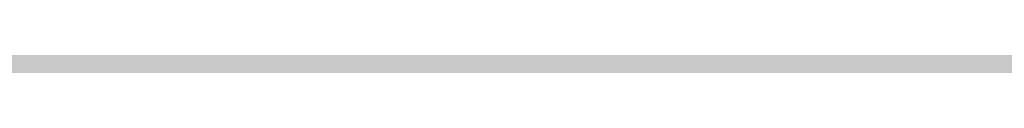
# Model space of a CAD drawing. Units: inches. Extents: x 2091 to 2899, y 967 to 2217.
# Tile 196 of 256: x 2203.18039 to 2203.25707, y 1152.24727 to 1152.24748. Entities that reach past the tile are written whole.
import ezdxf

# ---------------------------------------------------------------- set-up
doc = ezdxf.new("R2010")
doc.units = ezdxf.units.IN
doc.layers.add('A-WALL-PATT', color=141, linetype='Continuous', lineweight=13, true_color=0xadddf7)

msp = doc.modelspace()

# ---------------------------------------------------------------- hatches: boundary and pattern name
at = {"layer": 'A-WALL-PATT'}
h = msp.add_hatch(color=256, dxfattribs=at)
h.dxf.hatch_style = 1
h.paths.add_polyline_path([(2803.143603, 2050.919059), (2203.143603, 2050.919059), (2203.143603, 1090.919059), (2803.143603, 1090.919059)])
h.paths.add_polyline_path([(2635.79885, 1147.540465), (2674.524052, 1147.540465, 0.376086), (2678.529665, 1152.880202), (2678.529665, 1159.556473, 0.333335), (2674.524319, 1163.561846), (2674.524319, 1163.56185), (2674.524319, 1192.93439), (2635.805971, 1192.93439), (2597.087622, 1192.93439), (2597.087622, 1163.561846, 0.333335), (2593.082276, 1159.556473), (2593.082276, 1152.880202, 0.376086), (2597.087889, 1147.540465)], flags=0)
h.paths.add_polyline_path([(2436.010433, 1278.240778, 0.000483), (2435.952643, 1278.215027, -0.001328), (2435.935625, 1278.111693, -0.001711), (2436.11644, 1278.040758, 0.002185)], flags=0)
h.paths.add_polyline_path([(2794.143603, 1143.419059), (2794.143603, 1347.419059), (2543.370171, 1347.419059), (2543.370171, 1351.919059), (2794.143603, 1351.919059), (2794.143603, 1392.713555), (2793.947398, 1392.713555), (2793.947398, 1473.5369), (2794.143603, 1473.5369), (2794.143603, 1531.919059), (2650.143603, 1531.919059), (2650.143603, 1536.419059), (2794.143603, 1536.419059), (2794.143603, 1692.419059), (2609.375609, 1692.419059), (2609.375609, 1644.419059), (2604.875609, 1644.419059), (2604.875609, 1744.919059), (2609.375609, 1744.919059), (2609.375609, 1696.919059), (2794.143603, 1696.919059), (2794.143603, 1780.919059), (2609.643603, 1780.919059), (2493.875609, 1780.919059), (2493.875609, 1785.419059), (2609.643603, 1785.419059), (2794.143603, 1785.419059), (2794.143603, 1847.938821), (2793.951222, 1847.938821), (2793.951222, 1928.762166), (2794.143603, 1928.762166), (2794.143603, 1941.419059), (2614.143603, 1941.419059), (2614.143603, 1821.419059), (2609.643603, 1821.419059), (2609.643603, 1941.419059), (2392.143603, 1941.419059), (2392.143603, 1819.919059), (2387.643603, 1819.919059), (2387.643603, 1941.419059), (2212.143603, 1941.419059), (2212.143603, 1783.919059), (2392.143603, 1783.919059), (2392.143603, 1780.919059), (2212.143603, 1780.919059), (2212.143603, 1629.419059), (2387.643603, 1629.419059), (2387.643603, 1744.919059), (2392.143603, 1744.919059), (2392.143603, 1627.919059), (2317.143603, 1627.919059), (2317.143603, 1551.419059), (2317.143603, 1536.419059), (2459.383591, 1536.419059), (2459.383591, 1602.39648), (2463.883591, 1602.39648), (2463.883591, 1531.919059), (2456.643603, 1531.919059), (2456.643603, 1529.919059), (2452.143603, 1529.919059), (2452.143603, 1531.919059), (2312.643603, 1531.919059), (2312.643603, 1551.419059), (2306.143603, 1551.419059), (2306.143603, 1555.919059), (2308.143603, 1555.919059), (2308.143603, 1551.419059), (2312.643603, 1551.419059), (2312.643603, 1627.919059), (2212.143603, 1627.919059), (2212.143603, 1555.919059), (2270.143603, 1555.919059), (2270.143603, 1551.419059), (2212.143603, 1551.419059), (2212.143603, 1351.919059), (2272.143603, 1351.919059), (2272.143603, 1347.419059), (2212.143603, 1347.419059), (2212.143603, 1275.419059), (2308.143603, 1275.419059), (2308.143603, 1351.919059), (2452.143603, 1351.919059), (2452.143603, 1493.919059), (2456.643603, 1493.919059), (2456.643603, 1347.419059), (2312.643603, 1347.419059), (2312.643603, 1270.919059), (2212.143603, 1270.919059), (2212.143603, 1099.919059), (2281.237523, 1099.919059), (2282.871041, 1110.913803), (2282.008341, 1116.996603), (2278.557741, 1121.420403), (2268.205641, 1128.056203), (2272.087641, 1128.056203), (2273.812941, 1131.927003), (2279.420341, 1134.691903), (2285.027841, 1135.244903), (2287.615841, 1137.456803), (2288.047141, 1138.009803), (2289.341141, 1140.774703), (2291.066541, 1139.668703), (2292.360541, 1135.244903), (2295.379841, 1136.903803), (2296.242541, 1135.797903), (2297.105241, 1133.033003), (2300.124641, 1138.009803), (2303.143941, 1138.009803), (2304.437941, 1135.797903), (2303.143941, 1133.586003), (2306.594641, 1134.691903), (2307.888741, 1133.033003), (2310.908041, 1135.244903), (2313.927441, 1134.138903), (2315.62686, 1132.427102), (2308.320041, 1117.549603), (2290.203841, 1109.807903), (2288.909841, 1103.172103), (2289.272309, 1099.919059), (2434.918227, 1099.919059), (2431.593227, 1124.788059), (2429.930227, 1169.553059), (2430.927185, 1240.519694), (2435.658926, 1238.186126), (2437.135227, 1196.554059), (2438.798227, 1143.973059), (2442.678227, 1111.998059), (2446.558227, 1099.919059), (2794.143603, 1099.919059), (2794.143603, 1138.919059), (2548.032447, 1138.919059), (2548.032447, 1143.419059), (2548.032447, 1148.819059), (2546.668457, 1148.031559), (2528.685692, 1179.178622, 0.256256), (2512.032447, 1148.819059), (2512.032447, 1143.419059), (2512.032447, 1138.919059), (2507.532447, 1138.919059), (2507.532447, 1143.419059), (2507.532447, 1148.819059, 0.256256), (2490.879202, 1179.178622), (2472.896437, 1148.031559), (2471.532447, 1148.819059), (2471.532447, 1143.419059), (2467.032447, 1143.419059), (2467.032447, 1269.945786, 0.039061), (2460.909987, 1273.580059), (2467.032447, 1273.580059), (2467.032447, 1286.325364, 0.014511), (2465.216194, 1286.761905), (2467.032447, 1287.052576), (2467.032447, 1323.419059), (2471.532447, 1323.419059), (2471.532447, 1148.819059), (2489.532447, 1179.995973), (2490.896437, 1179.208473), (2490.879202, 1179.178622, -0.256256), (2507.532447, 1148.819059), (2507.532447, 1143.419059), (2512.032447, 1143.419059), (2512.032447, 1148.819059, -0.256256), (2528.685692, 1179.178622), (2528.668457, 1179.208473), (2530.032447, 1179.995973), (2548.032447, 1148.819059), (2548.032447, 1143.419059)], flags=16)
h.paths.add_polyline_path([(2607.768546, 1200.945083), (2607.768546, 1265.030625), (2597.087622, 1281.052011), (2619.784585, 1281.052011), (2627.795278, 1337.12686), (2635.79885, 1337.12686), (2643.816663, 1337.12686), (2651.827356, 1281.052011), (2674.524319, 1281.052011), (2663.843395, 1265.030625), (2663.843395, 1200.945083), (2635.805971, 1200.945083)], flags=0)
edge = h.paths.add_edge_path(flags=0)
edge.add_ellipse((13303.896215, 1272.998725), major_axis=(-10595.31304, 0.000001), ratio=0.842303870086, start_angle=0.6282372191, end_angle=0.6465540999, ccw=False)
edge.add_ellipse((2711.70045, 1156.852678), major_axis=(2.219769, 0), ratio=0.84230387, start_angle=111.535244, end_angle=180.628237, ccw=False)
edge.add_ellipse((13303.156292, 1272.998725), major_axis=(-10593.026306, 0), ratio=0.842303869544, start_angle=0.5282714718, end_angle=0.6465540971, ccw=False)
edge.add_line((2710.764596, 1175.333295), (2710.129986, 1175.333295))
edge.add_ellipse((2710.129986, 1176.579775), major_axis=(1.479846, 0), ratio=0.84230387, start_angle=180, end_angle=270, ccw=False)
edge.add_line((2708.65014, 1176.579775), (2708.65014, 1200.782914))
edge.add_ellipse((2710.129986, 1200.782914), major_axis=(1.479846, 0), ratio=0.84230387, start_angle=90, end_angle=180, ccw=False)
edge.add_line((2710.129986, 1202.029394), (2710.465075, 1202.029394))
edge.add_ellipse((13303.156292, 1272.998725), major_axis=(-10593.026306, 0), ratio=0.842303869544, start_angle=-0.0902290886, end_angle=0.3838667788, ccw=False)
edge.add_ellipse((2710.129986, 1290.927031), major_axis=(-1.479846, 0), ratio=0.84230387, start_angle=0, end_angle=90, ccw=False)
edge.add_line((2708.65014, 1290.927031), (2708.65014, 1315.13017))
edge.add_ellipse((2710.129986, 1315.13017), major_axis=(-1.479846, 0), ratio=0.84230387, start_angle=-90, end_angle=0, ccw=False)
edge.add_line((2710.129986, 1316.37665), (2710.706314, 1316.37665))
edge.add_ellipse((3238.40172, 1296.289566), major_axis=(528.234, 0), ratio=0.8423038695, start_angle=176.34957241, end_angle=177.82004969, ccw=False)
edge.add_ellipse((2775.063043, 1071.450696), major_axis=(313.307761, 0), ratio=0.8423038695, start_angle=102.12596555, end_angle=103.78052899, ccw=False)
edge.add_ellipse((2775.063043, 1078.305698), major_axis=(-305.302891, 0), ratio=0.8423038695, start_angle=-79.790461, end_angle=-77.55537271, ccw=False)
edge.add_ellipse((2695.141767, 1541.975383), major_axis=(-250.960216, 0), ratio=0.8423038695, start_angle=99.25656601, end_angle=102.55493264)
edge.add_line((2741.410326, 1334.214255), (2747.132545, 1337.378477))
edge.add_ellipse((2747.538616, 1336.857478), major_axis=(-0.739923, 0), ratio=0.8423039, start_angle=270, end_angle=307.93313, ccw=False)
edge.add_ellipse((2747.538616, 1336.857478), major_axis=(-0.739923, 0), ratio=0.8423039, start_angle=232.06687, end_angle=270, ccw=False)
edge.add_line((2747.944687, 1337.378477), (2753.666906, 1334.214255))
edge.add_ellipse((2799.935466, 1541.975383), major_axis=(250.960216, 0), ratio=0.8423038695, start_angle=257.44506736, end_angle=260.74343399)
edge.add_ellipse((2720.014189, 1078.305698), major_axis=(305.302891, 0), ratio=0.8423038695, start_angle=77.55537271, end_angle=79.790461, ccw=False)
edge.add_ellipse((2720.014189, 1071.450696), major_axis=(-313.307761, 0), ratio=0.8423038695, start_angle=256.21947101, end_angle=257.87403445, ccw=False)
edge.add_ellipse((2256.675512, 1296.289566), major_axis=(-528.234, 0), ratio=0.8423038695, start_angle=182.17995031, end_angle=183.65042759, ccw=False)
edge.add_line((2784.370918, 1316.37665), (2784.947247, 1316.37665))
edge.add_ellipse((2784.947247, 1315.13017), major_axis=(1.479846, 0), ratio=0.84230387, start_angle=0, end_angle=90, ccw=False)
edge.add_line((2786.427093, 1315.13017), (2786.427093, 1290.927031))
edge.add_ellipse((2784.947247, 1290.927031), major_axis=(1.479846, 0), ratio=0.84230387, start_angle=270, end_angle=360, ccw=False)
edge.add_ellipse((-7808.07906, 1272.998725), major_axis=(10593.026306, 0), ratio=0.842303869544, start_angle=-0.3838667788, end_angle=0.0902290886, ccw=False)
edge.add_line((2784.612157, 1202.029394), (2784.947247, 1202.029394))
edge.add_ellipse((2784.947247, 1200.782914), major_axis=(1.479846, 0), ratio=0.84230387, start_angle=0, end_angle=90, ccw=False)
edge.add_line((2786.427093, 1200.782914), (2786.427093, 1176.579775))
edge.add_ellipse((2784.947247, 1176.579775), major_axis=(-1.479846, 0), ratio=0.84230387, start_angle=90, end_angle=180, ccw=False)
edge.add_line((2784.947247, 1175.333295), (2784.312636, 1175.333295))
edge.add_ellipse((-7808.07906, 1272.998725), major_axis=(10593.026306, 0), ratio=0.842303869544, start_angle=-0.6186431963, end_angle=-0.5282714718, ccw=False)
edge.add_ellipse((2783.376783, 1156.852678), major_axis=(-2.219769, 0), ratio=0.84230387, start_angle=179.371763, end_angle=248.464757, ccw=False)
edge.add_ellipse((-7808.818983, 1272.998725), major_axis=(-10595.31304, 0.000004), ratio=0.842303865762, start_angle=179.3534459226, end_angle=179.3717628034, ccw=False)
edge.add_ellipse((2780.297303, 1153.500793), major_axis=(-5.246426, 0), ratio=0.84230387, start_angle=90, end_angle=179.353446, ccw=False)
edge.add_line((2780.297303, 1149.081708), (2714.77993, 1149.081708))
edge.add_ellipse((2714.77993, 1153.500793), major_axis=(5.246426, 0), ratio=0.84230387, start_angle=180.646554, end_angle=270, ccw=False)
edge = h.paths.add_edge_path(flags=0)
edge.add_line((2718.187367, 1151.007833), (2718.187367, 1170.472364))
edge.add_ellipse((2721.14706, 1170.472364), major_axis=(-2.959692, 0), ratio=0.84230387, start_angle=-90, end_angle=0, ccw=False)
edge.add_line((2721.14706, 1172.965324), (2773.930173, 1172.965324))
edge.add_ellipse((2773.930173, 1170.472364), major_axis=(-2.959692, 0), ratio=0.84230387, start_angle=180, end_angle=270, ccw=False)
edge.add_line((2776.889865, 1170.472364), (2776.889865, 1151.007833))
edge.add_line((2776.889865, 1151.007833), (2718.187367, 1151.007833))
edge = h.paths.add_edge_path(flags=0)
edge.add_line((2718.187367, 1180.23415), (2718.187367, 1199.057834))
edge.add_ellipse((2747.538616, 1320.39864), major_axis=(147.017924, 0), ratio=0.8423038695, start_angle=256.40186531, end_angle=283.59813469)
edge.add_line((2776.889865, 1199.057834), (2776.889865, 1180.23415))
edge.add_ellipse((2747.538616, 1301.574956), major_axis=(147.017924, 0), ratio=0.8423038695, start_angle=256.40186531, end_angle=283.59813469, ccw=False)
edge = h.paths.add_edge_path(flags=0)
edge.add_ellipse((13303.156292, 1272.998725), major_axis=(-10591.54646, 0), ratio=0.842303869555, start_angle=0.0555943135, end_angle=0.3777641939, ccw=False)
edge.add_line((2711.616859, 1262.72171), (2715.667408, 1249.495396))
edge.add_ellipse((6413.891963, 1241.691919), major_axis=(-3698.236159, 0), ratio=0.84230386955, start_angle=-0.120897369, end_angle=0.364076349)
edge.add_line((2715.761038, 1218.192455), (2711.934307, 1203.167361))
edge = h.paths.add_edge_path(flags=0)
edge.add_line((2718.187367, 1251.074566), (2716.002485, 1267.450435))
edge.add_ellipse((2742.151175, 1202.18954), major_axis=(81.772585, 0), ratio=0.84230387, start_angle=94.27742096, end_angle=111.8349538, ccw=False)
edge.add_line((2737.009748, 1270.930626), (2758.067484, 1270.930626))
edge.add_ellipse((2752.926058, 1202.18954), major_axis=(81.772585, 0), ratio=0.84230387, start_angle=68.1650462, end_angle=85.72257904, ccw=False)
edge.add_line((2779.074747, 1267.450435), (2776.889865, 1251.074566))
edge.add_ellipse((2750.338059, 1187.885356), major_axis=(79.579664, 0), ratio=0.84230387, start_angle=67.20808512, end_angle=85.1299304)
edge.add_line((2756.034656, 1254.743656), (2739.042576, 1254.743656))
edge.add_ellipse((2744.739174, 1187.885356), major_axis=(79.579664, 0), ratio=0.84230387, start_angle=94.8700696, end_angle=112.79191488)
edge = h.paths.add_edge_path(flags=0)
edge.add_line((2783.142926, 1203.167361), (2779.316194, 1218.192455))
edge.add_ellipse((-918.81473, 1241.691919), major_axis=(3698.236159, 0), ratio=0.84230386955, start_angle=-0.364076349, end_angle=0.120897369)
edge.add_line((2779.409825, 1249.495396), (2783.460373, 1262.72171))
edge.add_ellipse((-7808.07906, 1272.998725), major_axis=(-10591.54646, 0), ratio=0.84230386954, start_angle=179.6222358061, end_angle=179.9444056865, ccw=False)
edge = h.paths.add_edge_path(flags=0)
edge.add_ellipse((2734.200892, 1286.69044), major_axis=(-0.356609, 6.340078), ratio=0.60383358, start_angle=89.0020143, end_angle=253.657408, ccw=False)
edge.add_line((2730.369001, 1286.541806), (2730.369001, 1301.35198))
edge.add_line((2730.369001, 1301.35198), (2735.913311, 1305.214803))
edge.add_ellipse((2736.384917, 1304.734561), major_axis=(0.739923, 0), ratio=0.8423039, start_angle=90, end_angle=134.480211, ccw=False)
edge.add_line((2736.384917, 1305.357801), (2738.032783, 1305.357801))
edge.add_line((2738.032783, 1305.357801), (2738.032783, 1307.707927))
edge.add_ellipse((2794.201642, 1307.707927), major_axis=(56.168859, 0), ratio=0.84230387, start_angle=150.5614304, end_angle=180, ccw=False)
edge.add_ellipse((2700.875591, 1307.707927), major_axis=(-56.168859, 0), ratio=0.84230387, start_angle=180, end_angle=209.4385696, ccw=False)
edge.add_line((2757.04445, 1307.707927), (2757.04445, 1305.357801))
edge.add_line((2757.04445, 1305.357801), (2758.692316, 1305.357801))
edge.add_ellipse((2758.692316, 1304.734561), major_axis=(-0.739923, 0), ratio=0.8423039, start_angle=225.519789, end_angle=270, ccw=False)
edge.add_line((2759.163922, 1305.214803), (2764.708231, 1301.35198))
edge.add_line((2764.708231, 1301.35198), (2764.708231, 1286.541806))
edge.add_ellipse((2760.87634, 1286.69044), major_axis=(0.356609, 6.340078), ratio=0.60383358, start_angle=106.342592, end_angle=270.9979857, ccw=False)
edge.add_line((2757.04445, 1285.79709), (2757.04445, 1307.707927))
edge.add_ellipse((2700.875591, 1307.707927), major_axis=(-56.168859, 0), ratio=0.84230387, start_angle=180, end_angle=209.4385696)
edge.add_ellipse((2794.201642, 1307.707927), major_axis=(56.168859, 0), ratio=0.84230387, start_angle=150.5614304, end_angle=180)
edge.add_line((2738.032783, 1307.707927), (2738.032783, 1285.79709))
h.paths.add_polyline_path([(2417.812273, 1104.449704), (2413.492273, 1102.529704), (2410.612273, 1103.969704), (2409.172273, 1106.369704), (2407.252273, 1107.329704), (2406.292273, 1109.729704), (2405.332273, 1114.049704), (2405.332273, 1117.889704), (2406.292273, 1120.129704), (2407.252273, 1119.809704), (2408.848322, 1118.327658), (2410.173945, 1119.42417), (2410.211273, 1120.405704), (2411.040731, 1121.419054), (2410.699273, 1119.858704), (2410.173945, 1119.42417), (2410.088452, 1117.176109), (2411.132836, 1116.206324), (2413.972273, 1119.329704), (2416.852273, 1120.769704), (2416.869721, 1120.798784), (2417.035071, 1119.405116), (2417.896213, 1118.143384), (2418.292273, 1118.369704), (2419.544447, 1120.039269), (2419.360915, 1118.387487), (2419.032108, 1119.356151), (2418.398939, 1118.511926), (2419.252273, 1114.529704), (2418.794091, 1107.198795)], flags=0)
h.paths.add_polyline_path([(2508.870171, 1347.419059), (2508.370171, 1347.419059), (2508.370171, 1351.919059), (2508.870171, 1351.919059)], flags=0)
h.paths.add_polyline_path([(2473.370171, 1347.419059), (2472.370171, 1347.419059), (2467.870171, 1347.419059), (2467.870171, 1455.419059), (2472.370171, 1455.419059), (2472.370171, 1352.419059), (2473.370171, 1352.419059)], flags=0)
h.paths.add_polyline_path([(2352.106244, 1217.446197), (2349.226244, 1218.886197), (2347.786244, 1221.286197), (2345.866244, 1222.246197), (2344.906244, 1224.646197), (2343.946244, 1228.966197), (2343.946244, 1232.806197), (2344.906244, 1235.046197), (2345.866244, 1234.726197), (2347.462293, 1233.244152), (2348.787916, 1234.340663), (2348.825244, 1235.322197), (2349.654702, 1236.335547), (2349.313244, 1234.775197), (2348.787916, 1234.340663), (2348.702423, 1232.092603), (2349.746807, 1231.122817), (2352.586244, 1234.246197), (2355.466244, 1235.686197), (2355.483692, 1235.715277), (2355.649043, 1234.321609), (2356.510185, 1233.059877), (2356.906244, 1233.286197), (2358.158418, 1234.955762), (2357.974887, 1233.30398), (2357.646079, 1234.272644), (2357.012911, 1233.428419), (2357.866244, 1229.446197), (2357.408062, 1222.115288), (2356.426244, 1219.366197)], flags=0)
h.paths.add_polyline_path([(2348.2968, 1112.22442), (2347.0138, 1112.31042), (2345.5298, 1114.12742), (2345.7318, 1115.85842), (2346.8118, 1116.98242), (2346.8118, 1114.64642), (2345.8668, 1114.21442), (2346.8798, 1114.30042)], flags=0)
h.paths.add_polyline_path([(2347.0138, 1110.92642), (2346.2718, 1110.49342), (2346.6098, 1111.18642)], flags=0)
h.paths.add_polyline_path([(2345.8668, 1118.19442), (2345.5298, 1117.32942), (2343.7078, 1118.02142), (2344.3828, 1118.62642)], flags=0)
h.paths.add_polyline_path([(2346.6768, 1109.28242), (2346.0698, 1108.07142), (2345.8668, 1110.06142)], flags=0)
h.paths.add_polyline_path([(2345.0568, 1119.75142), (2343.6398, 1119.75142), (2343.9778, 1121.13542)], flags=0)
h.paths.add_polyline_path([(2345.2598, 1116.55042), (2345.1248, 1115.85842), (2344.9218, 1115.68542), (2344.7198, 1116.37742)], flags=0)
h.paths.add_polyline_path([(2345.6648, 1112.31042), (2345.4618, 1111.53242), (2344.0448, 1111.96442), (2344.6518, 1112.57042)], flags=0)
h.paths.add_polyline_path([(2345.1918, 1113.34942), (2344.4498, 1113.86842), (2344.7198, 1114.38742)], flags=0)
h.paths.add_polyline_path([(2344.6518, 1116.80942), (2344.1798, 1115.68542), (2344.6518, 1115.33942), (2343.9098, 1114.90642), (2343.0328, 1115.94442), (2343.6398, 1116.46342)], flags=0)
h.paths.add_polyline_path([(2345.8668, 1106.68642), (2344.9898, 1105.56242), (2344.5168, 1106.60042)], flags=0)
h.paths.add_polyline_path([(2344.8548, 1110.06142), (2344.5168, 1109.28242), (2344.1128, 1109.71542)], flags=0)
h.paths.add_polyline_path([(2344.0448, 1113.52242), (2343.4378, 1113.08942), (2342.7628, 1113.95442)], flags=0)
h.paths.add_polyline_path([(2344.3148, 1111.01242), (2342.9648, 1110.32042), (2342.9648, 1111.09942)], flags=0)
h.paths.add_polyline_path([(2345.1248, 1104.69742), (2344.5848, 1103.74542), (2344.4498, 1104.26442)], flags=0)
h.paths.add_polyline_path([(2342.8298, 1121.22242), (2341.7498, 1120.53042), (2340.5358, 1121.04942), (2340.1308, 1121.82842), (2340.6708, 1122.95242), (2341.1428, 1121.82842), (2341.6148, 1122.00142)], flags=0)
h.paths.add_polyline_path([(2342.9648, 1119.75142), (2343.0328, 1118.45342), (2342.0878, 1118.02142), (2342.0198, 1119.49142)], flags=0)
h.paths.add_polyline_path([(2342.6948, 1116.89642), (2341.9528, 1116.63642), (2342.0198, 1117.32942)], flags=0)
h.paths.add_polyline_path([(2343.0328, 1112.22442), (2342.0198, 1111.79142), (2341.5478, 1112.22442), (2342.3578, 1113.34942)], flags=0)
h.paths.add_polyline_path([(2343.7748, 1104.43742), (2342.6278, 1102.88042), (2342.6948, 1104.61042), (2343.4378, 1105.12942)], flags=0)
h.paths.add_polyline_path([(2342.0198, 1115.07942), (2340.8058, 1115.51242), (2340.9408, 1116.37742)], flags=0)
h.paths.add_polyline_path([(2341.4808, 1120.09742), (2341.4808, 1119.40542), (2341.0758, 1119.57842), (2341.1428, 1120.09742)], flags=0)
h.paths.add_polyline_path([(2341.8178, 1114.47342), (2340.9408, 1113.08942), (2340.8058, 1114.56042)], flags=0)
h.paths.add_polyline_path([(2341.1428, 1118.54042), (2340.9408, 1116.98242), (2339.0508, 1117.67542), (2339.0508, 1118.62642)], flags=0)
h.paths.add_polyline_path([(2342.6948, 1101.66842), (2341.9528, 1101.84142), (2342.5598, 1102.36142)], flags=0)
h.paths.add_polyline_path([(2340.3328, 1119.66542), (2338.4438, 1119.57842), (2337.9038, 1120.35742), (2339.6578, 1120.61642)], flags=0)
h.paths.add_polyline_path([(2340.3328, 1115.33942), (2340.0628, 1113.69542), (2339.3878, 1115.33942)], flags=0)
h.paths.add_polyline_path([(2341.8178, 1103.83142), (2341.5478, 1102.88042), (2341.1428, 1103.65842)], flags=0)
h.paths.add_polyline_path([(2339.0508, 1122.86642), (2337.2958, 1121.82842), (2337.0938, 1123.12542), (2337.7688, 1123.81842)], flags=0)
h.paths.add_polyline_path([(2339.1178, 1121.74142), (2338.8478, 1121.22242), (2338.1738, 1121.04942), (2338.3758, 1121.56842)], flags=0)
h.paths.add_polyline_path([(2339.1858, 1119.31942), (2338.6458, 1118.71342), (2338.2408, 1118.10742), (2338.2408, 1118.88642)], flags=0)
h.paths.add_polyline_path([(2341.1428, 1101.92842), (2340.6028, 1101.23642), (2340.0628, 1101.84142), (2340.6028, 1102.36142)], flags=0)
h.paths.add_polyline_path([(2337.6338, 1117.76142), (2336.6208, 1118.28042), (2337.2958, 1118.97242)], flags=0)
h.paths.add_polyline_path([(2336.8238, 1119.57842), (2334.7988, 1118.97242), (2335.2038, 1120.35742), (2336.5538, 1120.87642)], flags=0)
h.paths.add_polyline_path([(2339.1178, 1100.45742), (2337.3638, 1100.54342), (2336.7558, 1101.23642)], flags=0)
h.paths.add_polyline_path([(2336.3508, 1122.43342), (2336.0138, 1121.91442), (2334.9338, 1122.43342), (2334.5288, 1123.47142), (2335.7438, 1122.77942)], flags=0)
h.paths.add_polyline_path([(2334.7318, 1120.87642), (2334.2588, 1120.35742), (2334.0568, 1120.78942), (2334.5968, 1121.30842)], flags=0)
h.paths.add_polyline_path([(2334.4618, 1122.17442), (2332.5718, 1121.30842), (2331.3568, 1122.17442), (2332.0998, 1122.86642)], flags=0)
h.paths.add_polyline_path([(2334.2588, 1118.54042), (2333.3818, 1118.45342), (2333.6518, 1119.31942)], flags=0)
h.paths.add_polyline_path([(2335.5418, 1102.27442), (2334.1918, 1102.62042), (2335.2718, 1103.31242)], flags=0)
h.paths.add_polyline_path([(2332.7068, 1119.66542), (2331.6948, 1120.44342), (2332.5048, 1120.78942)], flags=0)
h.paths.add_polyline_path([(2334.7318, 1101.14942), (2333.5168, 1101.58242), (2333.9888, 1101.75542)], flags=0)
h.paths.add_polyline_path([(2332.6398, 1116.63642), (2331.0868, 1116.29042), (2331.9648, 1118.19442)], flags=0)
h.paths.add_polyline_path([(2330.7498, 1121.56842), (2330.2768, 1120.27042), (2328.5228, 1119.31942), (2328.9948, 1121.04942)], flags=0)
h.paths.add_polyline_path([(2330.7498, 1118.62642), (2330.0078, 1117.50242), (2329.8728, 1118.02142)], flags=0)
h.paths.add_polyline_path([(2332.0998, 1102.36142), (2330.5468, 1102.01442), (2331.6948, 1102.96642)], flags=0)
h.paths.add_polyline_path([(2329.5348, 1113.60842), (2329.0628, 1112.31042), (2328.5898, 1113.34942)], flags=0)
h.paths.add_polyline_path([(2328.3878, 1117.84842), (2327.5098, 1116.55042), (2327.1728, 1117.76142)], flags=0)
h.paths.add_polyline_path([(2329.7378, 1106.51342), (2329.5348, 1105.30242), (2328.2528, 1106.08142)], flags=0)
h.paths.add_polyline_path([(2328.6578, 1114.38742), (2328.0498, 1114.12742), (2328.3198, 1114.90642)], flags=0)
h.paths.add_polyline_path([(2328.3198, 1112.22442), (2327.1058, 1112.13742), (2326.7008, 1112.65642)], flags=0)
h.paths.add_polyline_path([(2326.9028, 1115.25242), (2326.7008, 1114.12742), (2325.2158, 1113.60842), (2326.0928, 1115.33942)], flags=0)
h.paths.add_polyline_path([(2326.6328, 1108.33042), (2326.0928, 1107.37942), (2325.8908, 1108.50342), (2326.4978, 1109.10942)], flags=0)
h.paths.add_polyline_path([(2615.143603, 1531.919059), (2609.643603, 1531.919059), (2609.643603, 1620.419059), (2614.143603, 1620.419059), (2614.143603, 1536.419059), (2615.143603, 1536.419059)], flags=0)
h.paths.add_polyline_path([(2545.143603, 1563.419059), (2464.143603, 1563.419059), (2464.143603, 1632.419059), (2509.143603, 1632.419059), (2509.143603, 1627.919059), (2509.143603, 1603.919059), (2468.643603, 1603.919059), (2468.643603, 1567.919059), (2540.643603, 1567.919059), (2540.643603, 1591.919059), (2545.143603, 1591.919059)], flags=0)
h.paths.add_polyline_path([(2388.969048, 1549.985735), (2357.434181, 1549.985735), (2357.434181, 1623.360778), (2399.362777, 1623.360778), (2435.689465, 1623.360778), (2435.592547, 1602.559273), (2435.592547, 1602.39648), (2388.969048, 1602.39648)], flags=0)
h.paths.add_polyline_path([(2388.880628, 1555.809151), (2374.904429, 1555.809151), (2374.904429, 1600.571564), (2374.904429, 1615.457645), (2406.350877, 1615.457645), (2406.350877, 1618.939431), (2412.174293, 1615.457645), (2406.350877, 1611.97586), (2406.350877, 1615.457645), (2388.880628, 1615.457645)], flags=0)
h.paths.add_polyline_path([(2568.875609, 1644.419059), (2453.375609, 1644.419059), (2453.375609, 1785.419059), (2457.875609, 1785.419059), (2457.875609, 1648.919059), (2568.875609, 1648.919059)], flags=0)
h.paths.add_polyline_path([(2212.143603, 1945.919059), (2212.143603, 2041.919059), (2794.143603, 2041.919059), (2794.143603, 1945.919059)], flags=16)
h.paths.add_polyline_path([(2271.082728, 1964.317238), (2776.852968, 1964.317238), (2776.852968, 2037.169623), (2271.082728, 2037.169623)], flags=8)
h.paths.add_polyline_path([(2380.649285, 1536.824144), (2461.040809, 1536.824144), (2461.040809, 1554.652587), (2380.649285, 1554.652587)], flags=8)
h.paths.add_polyline_path([(2240.755709, 1609.725451), (2309.185829, 1609.725451), (2309.185829, 1617.698204), (2240.755709, 1617.698204)], flags=8)
h.paths.add_polyline_path([(2212.677255, 1313.504102), (2282.59152, 1313.504102), (2282.59152, 1322.745239), (2212.677255, 1322.745239)], flags=8)
h.paths.add_polyline_path([(2457.111976, 1114.778574), (2558.481581, 1114.778574), (2558.481581, 1142.219682), (2457.111976, 1142.219682)], flags=8)
h.paths.add_polyline_path([(2473.442337, 1273.010067), (2604.641226, 1273.010067), (2604.641226, 1318.346935), (2473.442337, 1318.346935)], flags=8)
h.paths.add_polyline_path([(2638.876302, 1626.977432), (2684.250367, 1627.976738), (2684.038483, 1637.597494), (2638.664417, 1636.598188)], flags=8)
h.paths.add_polyline_path([(2537.590554, 1453.793447), (2628.389547, 1453.793447), (2628.389547, 1475.344811), (2537.590554, 1475.344811)], flags=8)
h.paths.add_polyline_path([(2504.137638, 1714.632397), (2554.647187, 1714.632397), (2554.647187, 1730.237712), (2504.137638, 1730.237712)], flags=8)
h.paths.add_polyline_path([(2487.501181, 1575.651872), (2535.097121, 1575.651872), (2535.097121, 1598.377646), (2487.501181, 1598.377646)], flags=8)
h.paths.add_polyline_path([(2709.0994, 1735.710278), (2740.016601, 1735.710278), (2740.016601, 1749.937641), (2709.0994, 1749.937641)], flags=8)
h.paths.add_polyline_path([(2442.438424, 1792.171657), (2564.728835, 1792.171657), (2564.728835, 1842.000163), (2442.438424, 1842.000163)], flags=8)
h.paths.add_polyline_path([(2655.815801, 1809.644076), (2789.520142, 1806.693796), (2790.084977, 1832.291638), (2656.380635, 1835.241918)], flags=8)
h.paths.add_polyline_path([(2234.842697, 1797.720143), (2368.592851, 1794.768852), (2369.160718, 1820.504132), (2235.410564, 1823.455423)], flags=8)
h.paths.add_polyline_path([(2245.138466, 1644.006335), (2398.427733, 1640.6239), (2398.994842, 1666.32482), (2245.705575, 1669.707255)], flags=8)
h.paths.add_polyline_path([(2306.142847, 1431.168519), (2413.768314, 1428.793687), (2414.333148, 1454.391529), (2306.707682, 1456.76636)], flags=8)
h.paths.add_polyline_path([(2306.834582, 1458.233145), (2393.380484, 1456.323449), (2393.932808, 1481.354358), (2307.386907, 1483.264054)], flags=8)

doc.saveas('drawing.dxf')
